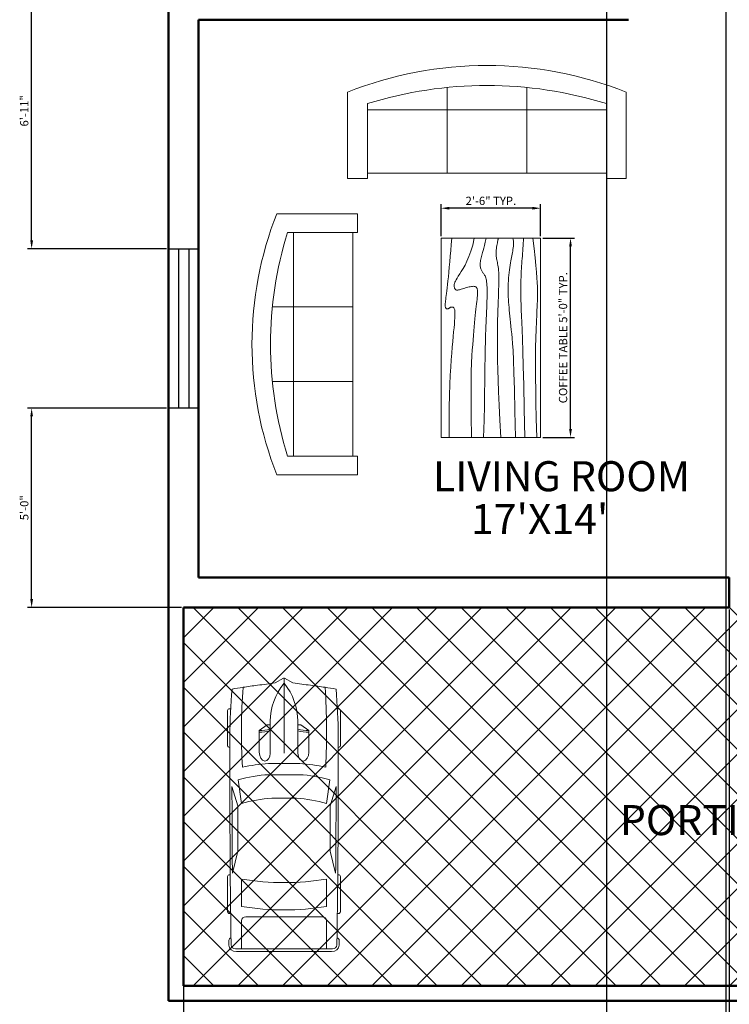
# Model space of a CAD drawing. Units: inches. Extents: x 2691 to 8091, y 3734 to 9067.
# Tile 2 of 5: x 2693 to 2906, y 3884 to 4181. Entities that reach past the tile are written whole.
import ezdxf

# ---------------------------------------------------------------- set-up
doc = ezdxf.new("R2010")
doc.units = ezdxf.units.IN
doc.layers.get('0').update_dxf_attribs({"color": 80})
for name, color, linetype, lineweight in [('A-ANNO-DIMS', 2, 'Continuous', 18), ('A-AREA-IDEN', 7, 'Continuous', 18), ('A-EQPM-VEH', 1, 'Continuous', 18), ('A-FLOR-PATT', 252, 'Continuous', 13), ('A-FURN', 8, 'Continuous', 18), ('A-WALL', 50, 'Continuous', 50), ('window', 4, 'Continuous', 25)]:
    doc.layers.add(name, color=color, linetype=linetype, lineweight=lineweight)
doc.styles.get("Standard").update_dxf_attribs({"font": 'arial.ttf'})
doc.dimstyles.new('ISO-25', dxfattribs={"dimtxt": 2.5, "dimasz": 2.5, "dimexe": 1.25, "dimexo": 0.625, "dimtad": 1, "dimdec": 1, "dimlunit": 3, "dimtxsty": 'Standard', "dimcen": 2.5, "dimadec": 0, "dimazin": 0, "dimtfac": 1, "dimtdec": 1, "dimtmove": 0, "dimatfit": 3, "dimfxl": 1, "dimarcsym": 0})

# ---------------------------------------------------------------- blocks, each defined once
blk = doc.blocks.new('Sofa - Roundback 7 ft.')
for p, q in [((-12.00002, -32.4421), (-12.00003, -6.5971)), ((11.99997, -32.4421), (11.99998, -6.5971)), ((-36.000027, -34), (-36.000027, -11.4696)), ((35.99998, -34), (35.99998, -11.4696)), ((-35.999844, -13.3819), (35.9998, -13.3819)), ((-36.000027, -32.4421), (35.99998, -32.4421))]:
    blk.add_line(p, q)
for points in [[(-36.000027, -34), (-42.000027, -34), (-42.000027, -8)], [(41.99998, -8), (41.99998, -34), (35.99998, -34)]]:
    blk.add_lwpolyline(points)
for centre, radius, start, end in [((0, -114.25), 114.25, 68.43141, 111.5686), ((-0.00001, -127.1968), 121.1968, 72.72033, 107.2797)]:
    blk.add_arc(centre, radius, start, end)
blk = doc.blocks.new('Table - Rectangular Woodgrain 60 x 30 in.')
for p, q in [((0, 0), (0, -30)), ((60, 0), (0, 0)), ((60, -30), (60, 0)), ((0, -30), (60, -30))]:
    blk.add_line(p, q)
for points in [[(0, -2.4), (4.8155, -2.418), (9.0302, -2.4688), (12.709, -2.5477), (15.9167, -2.65), (18.7181, -2.7711), (21.1781, -2.9063), (23.3616, -3.0508), (25.3333, -3.2), (27.1477, -3.3495), (28.8172, -3.4958), (30.3437, -3.636), (31.7291, -3.7667), (32.9756, -3.8849), (34.0849, -3.9875), (35.059, -4.0714), (35.9, -4.1334), (36.6114, -4.1711), (37.2041, -4.1854), (37.6906, -4.1779), (38.0833, -4.15), (38.3948, -4.1034), (38.6375, -4.0396), (38.8239, -3.9602), (38.9666, -3.8667), (39.0764, -3.7608), (39.1573, -3.6448), (39.2116, -3.521), (39.2416, -3.3917), (39.2498, -3.2593), (39.2385, -3.1261), (39.21, -2.9944), (39.1666, -2.8667), (39.111, -2.7447), (39.0468, -2.6281), (38.978, -2.5163), (38.9083, -2.4083), (38.8418, -2.3035), (38.7823, -2.201), (38.7337, -2.1001), (38.7, -2), (38.6844, -1.9003), (38.6875, -1.8021), (38.7094, -1.707), (38.75, -1.6167), (38.8094, -1.5326), (38.8875, -1.4563), (38.9844, -1.3893), (39.1, -1.3333), (39.2351, -1.2896), (39.3937, -1.2583), (39.5804, -1.2396), (39.8, -1.2333), (40.057, -1.2396), (40.3562, -1.2583), (40.7023, -1.2896), (41.1, -1.3333), (41.5547, -1.3895), (42.0755, -1.4573), (42.6721, -1.5361), (43.3542, -1.625), (44.1316, -1.7233), (45.014, -1.8302), (46.0114, -1.9449), (47.1333, -2.0667), (48.3862, -2.1947), (49.7625, -2.3281), (51.2513, -2.4663), (52.8416, -2.6083), (54.5226, -2.7535), (56.2833, -2.9011), (58.1127, -3.0501), (60, -3.2)], [(0, -9.2), (6.5759, -9.0858), (11.9385, -9.0365), (16.2527, -9.0418), (19.6833, -9.0917), (22.3952, -9.1759), (24.5531, -9.2844), (26.322, -9.4069), (27.8666, -9.5333), (29.3241, -9.6553), (30.7203, -9.7719), (32.0532, -9.8837), (33.3208, -9.9917), (34.5213, -10.0965), (35.6526, -10.199), (36.7128, -10.2999), (37.7, -10.4), (38.6129, -10.4996), (39.4531, -10.5969), (40.223, -10.6895), (40.925, -10.775), (41.5613, -10.8512), (42.1344, -10.9156), (42.6465, -10.966), (43.1, -11), (43.4976, -11.0158), (43.8437, -11.0136), (44.143, -10.9942), (44.4, -10.9583), (44.6195, -10.9069), (44.8062, -10.8406), (44.9648, -10.7603), (45.1, -10.6667), (45.2155, -10.5598), (45.3114, -10.4365), (45.3871, -10.2929), (45.4416, -10.125), (45.4743, -9.929), (45.4844, -9.7011), (45.4709, -9.4371), (45.4333, -9.1333), (45.3716, -8.7883), (45.2896, -8.4104), (45.1919, -8.0107), (45.0833, -7.6), (44.9685, -7.1893), (44.8521, -6.7896), (44.7388, -6.4117), (44.6333, -6.0667), (44.54, -5.7628), (44.4614, -5.4979), (44.4001, -5.2675), (44.3583, -5.0667), (44.3384, -4.8909), (44.3427, -4.7354), (44.3736, -4.5956), (44.4333, -4.4667), (44.5236, -4.3453), (44.6427, -4.2333), (44.7884, -4.1339), (44.9583, -4.05), (45.1501, -3.9849), (45.3614, -3.9417), (45.59, -3.9234), (45.8333, -3.9333), (46.0915, -3.9749), (46.3734, -4.0531), (46.6906, -4.1736), (47.0542, -4.3417), (47.4756, -4.5629), (47.9661, -4.8427), (48.5372, -5.1866), (49.2, -5.6), (49.9676, -6.0844), (50.8594, -6.625), (51.8965, -7.2031), (53.1, -7.8), (54.491, -8.3969), (56.0906, -8.975), (57.9199, -9.5156), (60, -10)], [(0, -12.8), (5.1847, -12.9322), (9.6213, -13.0323), (13.3963, -13.1059), (16.5958, -13.1583), (19.3063, -13.1952), (21.614, -13.2219), (23.6054, -13.2439), (25.3666, -13.2667), (26.9728, -13.2947), (28.4531, -13.3281), (29.8256, -13.3663), (31.1083, -13.4083), (32.3191, -13.4535), (33.476, -13.501), (34.597, -13.5501), (35.7, -13.6), (36.7984, -13.6497), (37.8875, -13.6979), (38.9578, -13.743), (40, -13.7833), (41.0047, -13.8174), (41.9625, -13.8438), (42.864, -13.8607), (43.7, -13.8667), (44.4631, -13.8604), (45.1552, -13.8417), (45.7801, -13.8104), (46.3416, -13.7667), (46.8439, -13.7104), (47.2906, -13.6417), (47.6858, -13.5604), (48.0333, -13.4667), (48.3375, -13.3608), (48.6042, -13.2448), (48.8396, -13.121), (49.05, -12.9917), (49.2417, -12.8593), (49.4208, -12.7261), (49.5937, -12.5944), (49.7667, -12.4667), (49.9452, -12.3451), (50.1323, -12.2313), (50.3303, -12.1268), (50.5416, -12.0333), (50.7686, -11.9524), (51.0135, -11.8854), (51.2788, -11.8341), (51.5666, -11.8), (51.8785, -11.7843), (52.2116, -11.7865), (52.562, -11.8059), (52.926, -11.8417), (53.2998, -11.8931), (53.6795, -11.9594), (54.0614, -12.0397), (54.4416, -12.1333), (54.8223, -12.2401), (55.2293, -12.3625), (55.6942, -12.5037), (56.2489, -12.6667), (56.9251, -12.8547), (57.7545, -13.0708), (58.7689, -13.3182), (60, -13.6)], [(0, -18), (5.124, -17.7273), (9.6609, -17.5057), (13.6705, -17.3303), (17.2125, -17.1958), (20.3467, -17.0973), (23.1328, -17.0297), (25.6307, -16.9878), (27.9, -16.9667), (29.9928, -16.9617), (31.9302, -16.9703), (33.7254, -16.9907), (35.3917, -17.0208), (36.9423, -17.0588), (38.3906, -17.1026), (39.7499, -17.1503), (41.0333, -17.2), (42.2519, -17.2496), (43.4073, -17.2969), (44.4986, -17.3395), (45.525, -17.375), (46.4858, -17.4012), (47.3802, -17.4156), (48.2074, -17.416), (48.9667, -17.4), (49.6583, -17.3662), (50.2872, -17.3167), (50.8595, -17.2547), (51.3812, -17.1833), (51.8584, -17.1057), (52.2971, -17.025), (52.7034, -16.9443), (53.0833, -16.8667), (53.443, -16.7951), (53.789, -16.7313), (54.128, -16.6768), (54.4666, -16.6334), (54.8115, -16.6024), (55.1693, -16.5854), (55.5465, -16.5841), (55.95, -16.6), (56.3828, -16.6337), (56.8346, -16.6823), (57.2915, -16.7418), (57.7396, -16.8084), (58.165, -16.878), (58.5539, -16.9469), (58.8924, -17.0111), (59.1666, -17.0667), (59.3679, -17.1107), (59.5078, -17.1438), (59.6032, -17.1675), (59.6708, -17.1833), (59.7275, -17.193), (59.7901, -17.1979), (59.8753, -17.1998), (60, -17.2)], [(0, -22.4), (8.0098, -22.2501), (14.4094, -22.1011), (19.4168, -21.9535), (23.25, -21.8083), (26.1269, -21.6663), (28.2656, -21.5281), (29.884, -21.3947), (31.2, -21.2667), (32.3967, -21.1448), (33.5172, -21.0292), (34.5697, -20.9198), (35.5625, -20.8167), (36.5037, -20.7198), (37.4015, -20.6292), (38.2642, -20.5448), (39.1, -20.4667), (39.9164, -20.3951), (40.7187, -20.3313), (41.5117, -20.2768), (42.3, -20.2333), (43.0883, -20.2024), (43.8812, -20.1854), (44.6836, -20.1841), (45.5, -20.2), (46.3328, -20.234), (47.1747, -20.2844), (48.0163, -20.3488), (48.8479, -20.425), (49.66, -20.5106), (50.4429, -20.6031), (51.1872, -20.7004), (51.8833, -20.8), (52.5246, -20.8999), (53.1166, -20.9995), (53.6681, -21.0983), (54.1875, -21.1958), (54.6834, -21.2919), (55.1646, -21.3859), (55.6394, -21.4777), (56.1167, -21.5667), (56.6028, -21.6515), (57.0961, -21.7266), (57.5929, -21.7852), (58.0896, -21.8208), (58.5823, -21.8268), (59.0674, -21.7964), (59.5412, -21.723), (60, -21.6)], [(0, -25.2), (8.6355, -25.0504), (15.7026, -24.9031), (21.4049, -24.7606), (25.9458, -24.625), (29.529, -24.4988), (32.3578, -24.3844), (34.6359, -24.284), (36.5667, -24.2), (38.3213, -24.1341), (39.9417, -24.0854), (41.437, -24.0523), (42.8167, -24.0333), (44.0901, -24.0268), (45.2667, -24.0313), (46.3557, -24.0451), (47.3667, -24.0667), (48.309, -24.0947), (49.1928, -24.1287), (50.0284, -24.168), (50.826, -24.2125), (51.5959, -24.2617), (52.3483, -24.3151), (53.0935, -24.3725), (53.8417, -24.4334), (54.6009, -24.497), (55.3699, -24.561), (56.1454, -24.6226), (56.9239, -24.6792), (57.7021, -24.7279), (58.4764, -24.7662), (59.2435, -24.7911), (60, -24.8)], [(0, -28.8), (5.6867, -28.6681), (10.45, -28.5698), (14.407, -28.5012), (17.675, -28.4584), (20.3711, -28.4374), (22.6125, -28.4344), (24.5164, -28.4455), (26.2, -28.4667), (27.762, -28.4947), (29.2276, -28.5281), (30.6033, -28.5663), (31.8958, -28.6084), (33.1118, -28.6535), (34.2578, -28.7011), (35.3405, -28.7501), (36.3666, -28.8), (37.3443, -28.8497), (38.288, -28.8974), (39.2137, -28.9412), (40.1375, -28.9792), (41.0753, -29.0093), (42.0432, -29.0297), (43.0572, -29.0384), (44.1333, -29.0333), (45.2936, -29.0114), (46.5843, -28.9641), (48.0579, -28.8816), (49.7666, -28.7542), (51.7629, -28.5721), (54.0989, -28.3255), (56.8272, -28.0048), (60, -27.6)]]:
    blk.add_lwpolyline(points)
blk = doc.blocks.new('Dining Set - 36 x 72 in')
at = {"layer": 'window'}
for p, q in [((418.4, 887.02), (466.4, 887.02)), ((418.4, 883.92), (466.4, 883.92))]:
    blk.add_line(p, q, dxfattribs=at)
blk.add_lwpolyline([(418.4, 881.14), (418.4, 890.14), (466.4, 890.14), (466.4, 881.14)], close=True, dxfattribs=at)
blk = doc.blocks.new('*U11')
for p, q in [((536, 950), (536, 936)), ((1182, 988), (568, 988)), ((1214, 950), (1214, 950)), ((2235, 810), (1899, 912)), ((3412, 904), (3030, 807)), ((3440, 942), (3440, 950)), ((3472, 988), (4087, 988)), ((4119, 950), (4119, 934)), ((1779, 801), (2195, 746)), ((3516, 746), (3994, 746)), ((4736, 746), (4242, 746)), ((4736, -851), (4736, 851)), ((4785, -832), (4785, 832)), ((4179, 670), (4179, -670)), ((820, 295), (918, 436)), ((918, 436), (1294, 436)), ((756, 241), (1313, 241)), ((816, 241), (816, 283)), ((1496, -274), (1496, 274)), ((1690, -267), (1690, 267)), ((2102, 216), (2102, -216)), ((4736, -267), (4736, 267)), ((83, 156), (3, 10)), ((0, 0), (1313, 0)), ((3, -10), (83, -156)), ((756, -241), (1313, -241)), ((816, -241), (816, -283)), ((820, -295), (918, -436)), ((918, -436), (1294, -436)), ((2195, -746), (1779, -801)), ((2235, -810), (1899, -912)), ((3412, -904), (3030, -807)), ((3994, -746), (3516, -746)), ((4242, -746), (4736, -746)), ((536, -950), (536, -936)), ((1182, -988), (568, -988)), ((1214, -950), (1214, -950)), ((3440, -942), (3440, -950)), ((3472, -988), (4087, -988)), ((4119, -950), (4119, -934))]:
    blk.add_line(p, q)
for centre, major_axis, ratio, start_param, end_param in [((6757, -699), (0, 7958), 0.842304, 1.367076, 1.39176), ((1046, -12468), (0, 13417), 0.842304, 0.00281, 0.075598), ((568, 950), (0, -37.6), 0.842304, 3.141593, 4.712389), ((1638, -268113), (0, 269063), 0.842304, -0.013397, 0.002797), ((1182, 950), (0, 37.6), 0.842304, -1.570796, 0), ((1638, -268113), (0, -269025), 0.842304, 3.133765, 3.140441), ((3472, 950), (0, -37.6), 0.842304, 3.141593, 4.712389), ((4087, 950), (0, 37.6), 0.842304, -1.570796, 0), ((4588, 910), (0, 56.4), 0.842304, -0.013017, 1.249894), ((1638, -268131), (0, 269121), 0.842304, -0.013397, -0.013017), ((4673, 851), (0, -75.2), 0.842304, 1.570796, 3.128196), ((4673, 832), (0, -133), 0.842304, 1.570796, 3.128196), ((6583, -699), (0, -7755), 0.842304, 4.528606, 4.561838), ((952, -15087), (0, -15833), 0.842304, 3.096046, 3.200911), ((3414, 137), (0, -2280), 0.842304, 4.449482, 4.652344), ((3436, 137), (0, 2077), 0.842304, 1.245306, 1.50788), ((3800, 71), (0, -2021), 0.842304, 4.372215, 4.640744), ((2433, -93125), (0, -93935), 0.842304, 3.134049, 3.144098), ((434, 0), (0, 3734), 0.842304, 4.511394, 4.913384), ((912, 0), (0, 3734), 0.842304, 4.511394, 4.913384), ((4242, 670), (0, 75.2), 0.842304, 0, 1.570796), ((-5194, 1331), (0, -6374), 0.842304, 1.385369, 1.434372), ((331, 432), (0, 696), 0.842304, 4.435146, 4.718221), ((361, 432), (0, 696), 0.842304, 4.435146, 4.718221), ((1290, 339), (161, -9), 0.603834, -1.395552, 1.581315), ((756, -1185), (0, 1427), 0.842304, 0, 0.590319), ((832, 283), (0, 18.8), 0.842304, 0.879714, 1.570796), ((16, 0), (0, -18.8), 0.842304, 4.131459, 5.293319), ((-5194, -1331), (0, 6374), 0.842304, -1.434372, -1.385369), ((756, 1185), (0, 1427), 0.842304, 2.551274, 3.141593), ((832, -283), (0, -18.8), 0.842304, 4.712389, 5.403472), ((331, -432), (0, -696), 0.842304, 1.564964, 1.848039), ((361, -432), (0, -696), 0.842304, 1.564964, 1.848039), ((3414, -137), (0, -2280), 0.842304, -1.510751, -1.307889), ((3436, -137), (0, -2077), 0.842304, -1.50788, -1.245306), ((3800, -71), (0, -2021), 0.842304, -1.499151, -1.230623), ((6583, 699), (0, 7755), 0.842304, 1.721348, 1.754579), ((4242, -670), (0, -75.2), 0.842304, 4.712389, 6.283185), ((6757, 699), (0, 7958), 0.842304, 1.749832, 1.774517), ((952, 15087), (0, -15833), 0.842304, -0.059319, 0.045547), ((2433, 93125), (0, -93935), 0.842304, -0.002505, 0.007544), ((4673, -851), (0, 75.2), 0.842304, 3.15499, 4.712389), ((4673, -832), (0, -133), 0.842304, 0.013397, 1.570796), ((1046, 12468), (0, -13417), 0.842304, -0.075598, -0.00281), ((568, -950), (0, 37.6), 0.842304, 1.570796, 3.141593), ((1638, 268113), (0, 269063), 0.842304, 3.138796, 3.15499), ((1182, -950), (0, -37.6), 0.842304, 0, 1.570796), ((1638, 268113), (0, -269025), 0.842304, 0.001152, 0.007828), ((3472, -950), (0, -37.6), 0.842304, -1.570796, 0), ((4087, -950), (0, 37.6), 0.842304, 3.141593, 4.712389), ((4588, -910), (0, -56.4), 0.842304, -1.249894, 0.013017), ((1638, 268131), (0, 269121), 0.842304, 3.15461, 3.15499)]:
    blk.add_ellipse(centre, major_axis=major_axis, ratio=ratio, start_param=start_param, end_param=end_param)
at = {"extrusion": (0, 0, -1)}
blk.add_ellipse((1290, -339), major_axis=(161, 9), ratio=0.603834, start_param=-1.395552, end_param=1.581315, dxfattribs=at)
blk = doc.blocks.new('*D37')
at = {"layer": 'A-ANNO-DIMS', "color": 0, "lineweight": -2, "transparency": 16777216}
for p, q in [((2850.24, 4115.04), (2859.86, 4115.04)), ((2858.61, 4057.54), (2858.61, 4112.54)), ((2850.24, 4055.04), (2859.86, 4055.04))]:
    blk.add_line(p, q, dxfattribs=at)
at = {"layer": 'A-ANNO-DIMS', "color": 0, "transparency": 16777216}
for points in [[(2858.19, 4112.54), (2859.03, 4112.54), (2858.61, 4115.04)], [(2858.19, 4057.54), (2859.03, 4057.54), (2858.61, 4055.04)]]:
    blk.add_solid(points, dxfattribs=at)
at = {"layer": 'Defpoints', "color": 0, "transparency": 16777216}
for p in [(2849.61, 4115.04), (2858.61, 4115.04), (2849.61, 4055.04)]:
    blk.add_point(p, dxfattribs=at)
at = {"layer": 'A-ANNO-DIMS', "color": 0, "transparency": 16777216, "insert": (2856.69, 4085.04), "char_height": 2.5, "attachment_point": 5, "rotation": 90}
blk.add_mtext('COFFEE TABLE 5\'-0" TYP.', dxfattribs=at)
blk = doc.blocks.new('*D38')
at = {"layer": 'A-ANNO-DIMS', "color": 0, "lineweight": -2, "transparency": 16777216}
for p, q in [((2819.61, 4115.66), (2819.61, 4125.29)), ((2849.61, 4115.66), (2849.61, 4125.29)), ((2847.11, 4124.04), (2822.11, 4124.04))]:
    blk.add_line(p, q, dxfattribs=at)
at = {"layer": 'A-ANNO-DIMS', "color": 0, "transparency": 16777216}
for points in [[(2822.11, 4124.46), (2822.11, 4123.62), (2819.61, 4124.04)], [(2847.11, 4124.46), (2847.11, 4123.62), (2849.61, 4124.04)]]:
    blk.add_solid(points, dxfattribs=at)
at = {"layer": 'Defpoints', "color": 0, "transparency": 16777216}
for p in [(2819.61, 4124.04), (2819.61, 4115.04), (2849.61, 4115.04)]:
    blk.add_point(p, dxfattribs=at)
at = {"layer": 'A-ANNO-DIMS', "color": 0, "transparency": 16777216, "insert": (2834.61, 4125.94), "char_height": 2.5, "attachment_point": 5}
blk.add_mtext('2\'-6" TYP.', dxfattribs=at)
blk = doc.blocks.new('*D49')
at = {"layer": 'A-ANNO-DIMS', "color": 0, "lineweight": -2, "transparency": 16777216}
for p, q in [((2736.83, 4194.89), (2694.95, 4194.89)), ((2696.2, 4114.35), (2696.2, 4192.39)), ((2736.83, 4111.85), (2694.95, 4111.85))]:
    blk.add_line(p, q, dxfattribs=at)
at = {"layer": 'A-ANNO-DIMS', "color": 0, "transparency": 16777216}
for points in [[(2695.79, 4192.39), (2696.62, 4192.39), (2696.2, 4194.89)], [(2695.79, 4114.35), (2696.62, 4114.35), (2696.2, 4111.85)]]:
    blk.add_solid(points, dxfattribs=at)
at = {"layer": 'Defpoints', "color": 0, "transparency": 16777216}
for p in [(2696.2, 4194.89), (2737.46, 4194.89), (2737.46, 4111.85)]:
    blk.add_point(p, dxfattribs=at)
at = {"layer": 'A-ANNO-DIMS', "color": 0, "transparency": 16777216, "insert": (2694.3, 4153.37), "char_height": 2.5, "attachment_point": 5, "rotation": 90}
blk.add_mtext('6\'-11"', dxfattribs=at)
blk = doc.blocks.new('*D50')
at = {"layer": 'A-ANNO-DIMS', "color": 0, "lineweight": -2, "transparency": 16777216}
for p, q in [((2736.83, 4063.85), (2694.95, 4063.85)), ((2696.2, 4006.32), (2696.2, 4061.35)), ((2741.33, 4003.82), (2694.95, 4003.82))]:
    blk.add_line(p, q, dxfattribs=at)
at = {"layer": 'A-ANNO-DIMS', "color": 0, "transparency": 16777216}
for points in [[(2695.79, 4061.35), (2696.62, 4061.35), (2696.2, 4063.85)], [(2695.79, 4006.32), (2696.62, 4006.32), (2696.2, 4003.82)]]:
    blk.add_solid(points, dxfattribs=at)
at = {"layer": 'Defpoints', "color": 0, "transparency": 16777216}
for p in [(2696.2, 4063.85), (2737.46, 4063.85), (2741.96, 4003.82)]:
    blk.add_point(p, dxfattribs=at)
at = {"layer": 'A-ANNO-DIMS', "color": 0, "transparency": 16777216, "insert": (2694.3, 4033.84), "char_height": 2.5, "attachment_point": 5, "rotation": 90}
blk.add_mtext('5\'-0"', dxfattribs=at)
blk = doc.blocks.new('*D56')
at = {"layer": 'A-ANNO-DIMS', "color": 0, "lineweight": -2, "transparency": 16777216}
for p, q in [((2741.96, 4003.19), (2741.96, 3735.06)), ((2906.46, 4003.19), (2906.46, 3735.06)), ((2744.46, 3736.31), (2903.96, 3736.31))]:
    blk.add_line(p, q, dxfattribs=at)
at = {"layer": 'A-ANNO-DIMS', "color": 0, "transparency": 16777216}
for points in [[(2744.46, 3736.72), (2744.46, 3735.89), (2741.96, 3736.31)], [(2903.96, 3736.72), (2903.96, 3735.89), (2906.46, 3736.31)]]:
    blk.add_solid(points, dxfattribs=at)
at = {"layer": 'Defpoints', "color": 0, "transparency": 16777216}
for p in [(2741.96, 4003.82), (2906.46, 4003.82), (2906.46, 3736.31)]:
    blk.add_point(p, dxfattribs=at)
at = {"layer": 'A-ANNO-DIMS', "color": 0, "transparency": 16777216, "insert": (2824.21, 3738.22), "char_height": 2.5, "attachment_point": 5}
blk.add_mtext('13\'-8 1/2"', dxfattribs=at)
blk = doc.blocks.new('*D57')
at = {"layer": 'A-ANNO-DIMS', "color": 0, "lineweight": -2, "transparency": 16777216}
for p, q in [((2906.46, 4003.19), (2906.46, 3735.06)), ((2947.46, 4003.19), (2947.46, 3735.06)), ((2908.96, 3736.31), (2944.96, 3736.31))]:
    blk.add_line(p, q, dxfattribs=at)
at = {"layer": 'A-ANNO-DIMS', "color": 0, "transparency": 16777216}
for points in [[(2908.96, 3736.72), (2908.96, 3735.89), (2906.46, 3736.31)], [(2944.96, 3736.72), (2944.96, 3735.89), (2947.46, 3736.31)]]:
    blk.add_solid(points, dxfattribs=at)
at = {"layer": 'Defpoints', "color": 0, "transparency": 16777216}
for p in [(2906.46, 4003.82), (2947.46, 4003.82), (2947.46, 3736.31)]:
    blk.add_point(p, dxfattribs=at)
at = {"layer": 'A-ANNO-DIMS', "color": 0, "transparency": 16777216, "insert": (2926.96, 3738.21), "char_height": 2.5, "attachment_point": 5}
blk.add_mtext('3\'-5"', dxfattribs=at)
blk = doc.blocks.new('*D59')
at = {"layer": 'A-ANNO-DIMS', "color": 0, "lineweight": -2, "transparency": 16777216}
for p, q in [((2869.46, 4415.69), (2869.46, 3735.06)), ((2905.46, 4415.69), (2905.46, 3735.06)), ((2871.96, 3736.31), (2902.96, 3736.31))]:
    blk.add_line(p, q, dxfattribs=at)
at = {"layer": 'A-ANNO-DIMS', "color": 0, "transparency": 16777216}
for points in [[(2871.96, 3736.72), (2871.96, 3735.89), (2869.46, 3736.31)], [(2902.96, 3736.72), (2902.96, 3735.89), (2905.46, 3736.31)]]:
    blk.add_solid(points, dxfattribs=at)
at = {"layer": 'Defpoints', "color": 0, "transparency": 16777216}
for p in [(2869.46, 4416.32), (2905.46, 4416.32), (2905.46, 3736.31)]:
    blk.add_point(p, dxfattribs=at)
at = {"layer": 'A-ANNO-DIMS', "color": 0, "transparency": 16777216, "insert": (2887.46, 3738.21), "char_height": 2.5, "attachment_point": 5}
blk.add_mtext('3\'-0"', dxfattribs=at)

msp = doc.modelspace()

# ---------------------------------------------------------------- hatches: boundary and pattern name
at = {"layer": 'A-FLOR-PATT'}
h = msp.add_hatch(dxfattribs=at)
h.set_pattern_fill('ANSI37', color=256, scale=3)
h.paths.add_polyline_path([(3079.46, 4003.82), (2741.96, 4003.82), (2741.96, 3889.82), (3079.46, 3889.82)])

# ---------------------------------------------------------------- linework, layer by layer
at = {"layer": 'A-WALL'}
for p, q in [((2737.46, 4597.82), (2737.46, 3885.32)), ((2746.46, 4180.82), (2876.06, 4180.82)), ((2746.46, 4180.82), (2746.46, 4012.82)), ((2746.46, 4012.82), (2906.46, 4012.82)), ((2906.46, 4012.82), (2906.46, 4003.82)), ((2741.96, 4003.82), (2906.46, 4003.82)), ((2741.96, 4003.82), (2741.96, 3889.82)), ((2741.96, 3889.82), (3079.46, 3889.82)), ((2737.46, 3885.32), (3083.96, 3885.32))]:
    msp.add_line(p, q, dxfattribs=at)

# ---------------------------------------------------------------- block references
at = {"layer": 'A-EQPM-VEH', "xscale": 0.0172096829913236, "yscale": 0.0172096829913236, "zscale": 0.0172096829913236, "rotation": 270}
msp.add_blockref('*U11', (2772.27, 3982.53), dxfattribs=at)
at = {"layer": 'A-FURN'}
msp.add_blockref('Sofa - Roundback 7 ft.', (2833.42, 4167.01), dxfattribs=at)
at = {"layer": 'A-FURN', "xscale": 0.9357531878624332, "yscale": 0.9357531878624332, "zscale": 0.9357531878624332, "rotation": 90}
msp.add_blockref('Sofa - Roundback 7 ft.', (2762.6, 4083.07), dxfattribs=at)
at = {"layer": 'A-FURN', "rotation": 90}
msp.add_blockref('Table - Rectangular Woodgrain 60 x 30 in.', (2819.61, 4055.04), dxfattribs=at)
at = {"layer": 'window', "rotation": 90}
msp.add_blockref('Dining Set - 36 x 72 in', (3627.6, 3645.45), dxfattribs=at)

# ---------------------------------------------------------------- texts
at = {"layer": 'A-AREA-IDEN'}
for s, height, p in [('LIVING ROOM', 9.0539, (2817.17, 4038.81)), ("17'X14'", 9.054, (2828.64, 4025.91)), ('PORTICO PARKING', 9.0539, (2873.51, 3935.24))]:
    msp.add_text(s, height=height, dxfattribs=at).set_placement(p)

# ---------------------------------------------------------------- dimensions: what is measured, and where the dimension line sits
at = {"layer": 'A-ANNO-DIMS'}
for base, p1, p2, picture, middle in [((2905.46, 3736.31), (2869.46, 4416.32), (2905.46, 4416.32), '*D59', (2887.46, 3738.21)), ((2906.46, 3736.31), (2741.96, 4003.82), (2906.46, 4003.82), '*D56', (2824.21, 3738.22)), ((2947.46, 3736.31), (2906.46, 4003.82), (2947.46, 4003.82), '*D57', (2926.96, 3738.21))]:
    dim = msp.add_linear_dim(base=base, p1=p1, p2=p2, dimstyle='ISO-25', override={"dimdec": 1, "dimlfac": 1, "dimrnd": 0, "dimzin": 1, "dimdsep": 46, "dimlunit": 4, "dimfrac": 2}, dxfattribs=at)
    dim.commit()
    dim.dimension.update_dxf_attribs({"geometry": picture, "text_midpoint": middle})
for base, p1, p2, picture, middle in [((2696.2, 4194.89), (2737.46, 4111.85), (2737.46, 4194.89), '*D49', (2694.3, 4153.37)), ((2696.2, 4063.85), (2741.96, 4003.82), (2737.46, 4063.85), '*D50', (2694.3, 4033.84))]:
    dim = msp.add_linear_dim(base=base, p1=p1, p2=p2, angle=90, dimstyle='ISO-25', override={"dimdec": 1, "dimlfac": 1, "dimrnd": 0, "dimzin": 1, "dimdsep": 46, "dimlunit": 4, "dimfrac": 2}, dxfattribs=at)
    dim.commit()
    dim.dimension.update_dxf_attribs({"geometry": picture, "text_midpoint": middle})
for base, p1, p2, angle, text, picture, middle in [((2819.61, 4124.04), (2849.61, 4115.04), (2819.61, 4115.04), 180, '<> TYP.', '*D38', (2834.61, 4125.94)), ((2858.61, 4115.04), (2849.61, 4055.04), (2849.61, 4115.04), 90, 'COFFEE TABLE <> TYP.', '*D37', (2856.69, 4085.04))]:
    dim = msp.add_linear_dim(base=base, p1=p1, p2=p2, angle=angle, text=text, dimstyle='ISO-25', override={"dimdec": 1, "dimlfac": 1, "dimrnd": 0, "dimzin": 1, "dimdsep": 46, "dimlunit": 4, "dimfrac": 2}, dxfattribs=at)
    dim.commit()
    dim.dimension.update_dxf_attribs({"geometry": picture, "text_midpoint": middle})

doc.saveas('drawing.dxf')
